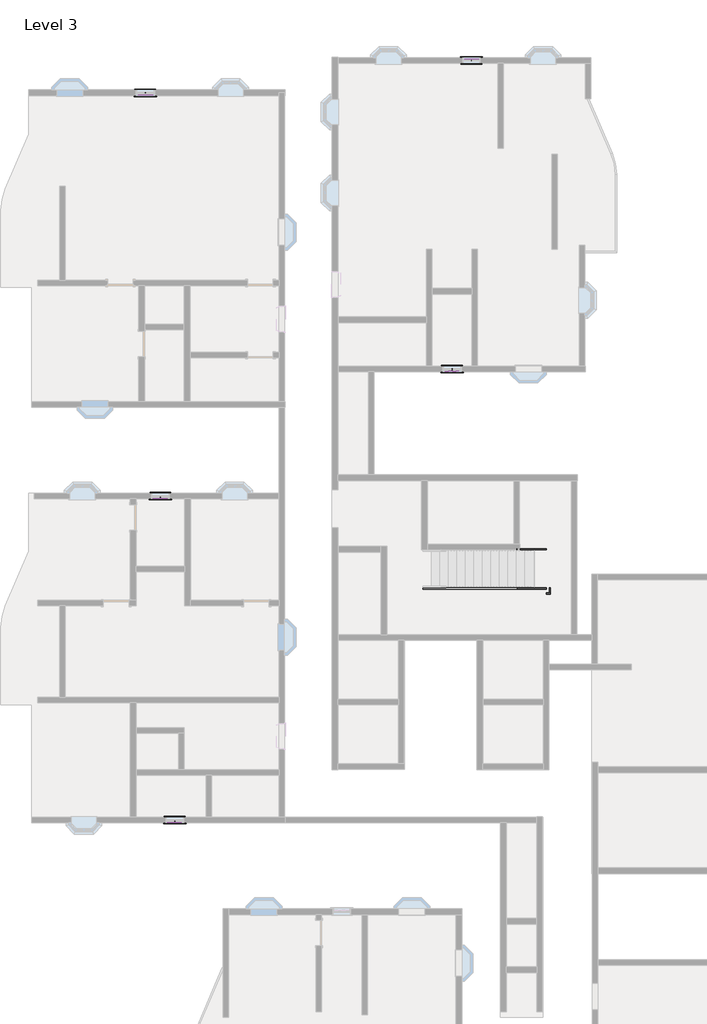
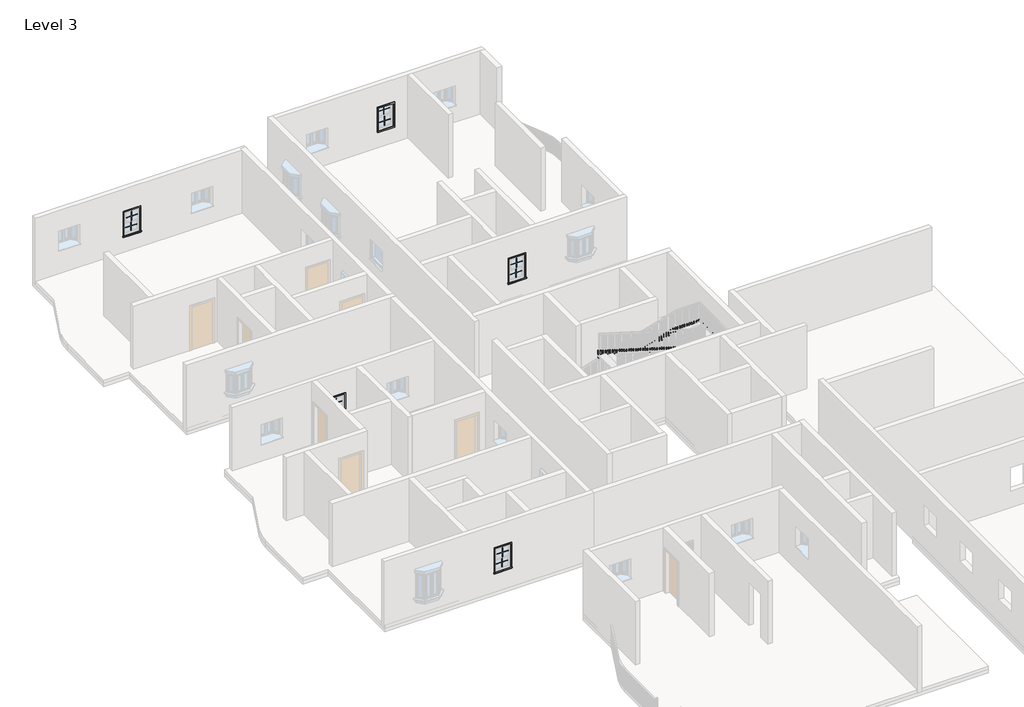
# One storey, part 14 of 14: 20 proxies, 6 members.
"""IFC4 building model written with IfcOpenShell, lengths in millimetres."""

from ifc_helpers import new_model, si_unit, frame, origin, place, context, project, spatial, polyline, outline, extrude, transform, mapped, element, save
from components import muntin_pattern_2x2_muntin_pattern_2x2_c35c595f, trim_window_exterior_flat_with_sill_e38017c9, trim_window_interior_flat_picture_frame_d728ed12

model = new_model("IFC4")

# Units and contexts
model_context = context("Model", 3, world=origin())
ifc_project = project(units=[si_unit("LENGTHUNIT", "METRE", prefix="MILLI")], contexts=[model_context])

# Site, building, storey
site = spatial("IfcSite", under=ifc_project)
building = spatial("IfcBuilding", under=site)
storey = spatial("IfcBuildingStorey", under=building, Name="Level 3", Elevation=6096.0)

# Proxies
placement = place(None, origin())
muntin_pattern_2x2_muntin_pattern_2x2_shape = muntin_pattern_2x2_muntin_pattern_2x2_c35c595f(model_context)
element("IfcBuildingElementProxy", 1, Name="Muntin Pattern_2x2 : Muntin Pattern_2x2", ObjectType="Muntin Pattern_2x2 : Muntin Pattern_2x2", at=placement, inside=storey, context=model_context, shape_type="MappedRepresentation", body=[
    mapped(muntin_pattern_2x2_muntin_pattern_2x2_shape, transform((-14639.3891351, 14368.0833494, 7566.025), x_axis=(-1.0, 0.0, 0.0), y_axis=(0.0, -1.0, 0.0), z_axis=(0.0, 0.0, 1.0))),
])
element("IfcBuildingElementProxy", 2, Name="Muntin Pattern_2x2 : Muntin Pattern_2x2", ObjectType="Muntin Pattern_2x2 : Muntin Pattern_2x2", at=placement, inside=storey, context=model_context, shape_type="MappedRepresentation", body=[
    mapped(muntin_pattern_2x2_muntin_pattern_2x2_shape, transform((-14639.3891351, 14412.5333494, 7086.6), x_axis=(-1.0, 0.0, 0.0), y_axis=(0.0, -1.0, 0.0), z_axis=(0.0, 0.0, 1.0))),
])
element("IfcBuildingElementProxy", 3, Name="Muntin Pattern_2x2 : Muntin Pattern_2x2", ObjectType="Muntin Pattern_2x2 : Muntin Pattern_2x2", at=placement, inside=storey, context=model_context, shape_type="MappedRepresentation", body=[
    mapped(muntin_pattern_2x2_muntin_pattern_2x2_shape, transform((-14125.0391351, 2785.6833494, 7566.025), x_axis=(-1.0, 0.0, 0.0), y_axis=(0.0, -1.0, 0.0), z_axis=(0.0, 0.0, 1.0))),
])
element("IfcBuildingElementProxy", 4, Name="Muntin Pattern_2x2 : Muntin Pattern_2x2", ObjectType="Muntin Pattern_2x2 : Muntin Pattern_2x2", at=placement, inside=storey, context=model_context, shape_type="MappedRepresentation", body=[
    mapped(muntin_pattern_2x2_muntin_pattern_2x2_shape, transform((-14125.0391351, 2830.1333494, 7086.6), x_axis=(-1.0, 0.0, 0.0), y_axis=(0.0, -1.0, 0.0), z_axis=(0.0, 0.0, 1.0))),
])
element("IfcBuildingElementProxy", 5, Name="Muntin Pattern_2x2 : Muntin Pattern_2x2", ObjectType="Muntin Pattern_2x2 : Muntin Pattern_2x2", at=placement, inside=storey, context=model_context, shape_type="MappedRepresentation", body=[
    mapped(muntin_pattern_2x2_muntin_pattern_2x2_shape, transform((-4206.3391351, 18910.0465905, 7566.025), x_axis=(-1.0, 0.0, 0.0), y_axis=(0.0, -1.0, 0.0), z_axis=(0.0, 0.0, 1.0))),
])
element("IfcBuildingElementProxy", 6, Name="Muntin Pattern_2x2 : Muntin Pattern_2x2", ObjectType="Muntin Pattern_2x2 : Muntin Pattern_2x2", at=placement, inside=storey, context=model_context, shape_type="MappedRepresentation", body=[
    mapped(muntin_pattern_2x2_muntin_pattern_2x2_shape, transform((-4206.3391351, 18954.4965905, 7086.6), x_axis=(-1.0, 0.0, 0.0), y_axis=(0.0, -1.0, 0.0), z_axis=(0.0, 0.0, 1.0))),
])
element("IfcBuildingElementProxy", 7, Name="Muntin Pattern_2x2 : Muntin Pattern_2x2", ObjectType="Muntin Pattern_2x2 : Muntin Pattern_2x2", at=placement, inside=storey, context=model_context, shape_type="MappedRepresentation", body=[
    mapped(muntin_pattern_2x2_muntin_pattern_2x2_shape, transform((-3514.1891351, 30066.9965905, 7566.025), x_axis=(1.0, 0.0, 0.0), y_axis=(0.0, 1.0, 0.0), z_axis=(0.0, 0.0, 1.0))),
])
element("IfcBuildingElementProxy", 8, Name="Muntin Pattern_2x2 : Muntin Pattern_2x2", ObjectType="Muntin Pattern_2x2 : Muntin Pattern_2x2", at=placement, inside=storey, context=model_context, shape_type="MappedRepresentation", body=[
    mapped(muntin_pattern_2x2_muntin_pattern_2x2_shape, transform((-3514.1891351, 30022.5465905, 7086.6), x_axis=(1.0, 0.0, 0.0), y_axis=(0.0, 1.0, 0.0), z_axis=(0.0, 0.0, 1.0))),
])
element("IfcBuildingElementProxy", 9, Name="Muntin Pattern_2x2 : Muntin Pattern_2x2", ObjectType="Muntin Pattern_2x2 : Muntin Pattern_2x2", at=placement, inside=storey, context=model_context, shape_type="MappedRepresentation", body=[
    mapped(muntin_pattern_2x2_muntin_pattern_2x2_shape, transform((-15175.9641351, 28782.5833494, 7566.025), x_axis=(-1.0, 0.0, 0.0), y_axis=(0.0, -1.0, 0.0), z_axis=(0.0, 0.0, 1.0))),
])
element("IfcBuildingElementProxy", 10, Name="Muntin Pattern_2x2 : Muntin Pattern_2x2", ObjectType="Muntin Pattern_2x2 : Muntin Pattern_2x2", at=placement, inside=storey, context=model_context, shape_type="MappedRepresentation", body=[
    mapped(muntin_pattern_2x2_muntin_pattern_2x2_shape, transform((-15175.9641351, 28827.0333494, 7086.6), x_axis=(-1.0, 0.0, 0.0), y_axis=(0.0, -1.0, 0.0), z_axis=(0.0, 0.0, 1.0))),
])
trim_window_exterior_flat_with_sill_shape = trim_window_exterior_flat_with_sill_e38017c9(model_context)
element("IfcBuildingElementProxy", 11, Name="Trim-Window-Exterior-Flat : with Sill", ObjectType="Trim-Window-Exterior-Flat : with Sill", at=placement, inside=storey, context=model_context, shape_type="MappedRepresentation", body=[
    mapped(trim_window_exterior_flat_with_sill_shape, transform((-14639.3891351, 14333.1583494, 8077.2), x_axis=(1.0, 0.0, 0.0), y_axis=(0.0, 0.0, 1.0), z_axis=(0.0, -1.0, 0.0))),
])
element("IfcBuildingElementProxy", 12, Name="Trim-Window-Exterior-Flat : with Sill", ObjectType="Trim-Window-Exterior-Flat : with Sill", at=placement, inside=storey, context=model_context, shape_type="MappedRepresentation", body=[
    mapped(trim_window_exterior_flat_with_sill_shape, transform((-14125.0391351, 2750.7583494, 8077.2), x_axis=(1.0, 0.0, 0.0), y_axis=(0.0, 0.0, 1.0), z_axis=(0.0, -1.0, 0.0))),
])
element("IfcBuildingElementProxy", 13, Name="Trim-Window-Exterior-Flat : with Sill", ObjectType="Trim-Window-Exterior-Flat : with Sill", at=placement, inside=storey, context=model_context, shape_type="MappedRepresentation", body=[
    mapped(trim_window_exterior_flat_with_sill_shape, transform((-4206.3391351, 18875.1215905, 8077.2), x_axis=(1.0, 0.0, 0.0), y_axis=(0.0, 0.0, 1.0), z_axis=(0.0, -1.0, 0.0))),
])
element("IfcBuildingElementProxy", 14, Name="Trim-Window-Exterior-Flat : with Sill", ObjectType="Trim-Window-Exterior-Flat : with Sill", at=placement, inside=storey, context=model_context, shape_type="MappedRepresentation", body=[
    mapped(trim_window_exterior_flat_with_sill_shape, transform((-3514.1891351, 30101.9215905, 8077.2), x_axis=(-1.0, 0.0, 0.0), y_axis=(0.0, 0.0, 1.0), z_axis=(0.0, 1.0, 0.0))),
])
element("IfcBuildingElementProxy", 15, Name="Trim-Window-Exterior-Flat : with Sill", ObjectType="Trim-Window-Exterior-Flat : with Sill", at=placement, inside=storey, context=model_context, shape_type="MappedRepresentation", body=[
    mapped(trim_window_exterior_flat_with_sill_shape, transform((-15175.9641351, 28747.6583494, 8077.2), x_axis=(1.0, 0.0, 0.0), y_axis=(0.0, 0.0, 1.0), z_axis=(0.0, -1.0, 0.0))),
])
trim_window_interior_flat_picture_frame_shape = trim_window_interior_flat_picture_frame_d728ed12(model_context)
element("IfcBuildingElementProxy", 16, Name="Trim-Window-Interior-Flat : Picture Frame", ObjectType="Trim-Window-Interior-Flat : Picture Frame", at=placement, inside=storey, context=model_context, shape_type="MappedRepresentation", body=[
    mapped(trim_window_interior_flat_picture_frame_shape, transform((-14639.3891351, 14536.3583494, 8077.2), x_axis=(-1.0, 0.0, 0.0), y_axis=(0.0, 0.0, 1.0), z_axis=(0.0, 1.0, 0.0))),
])
element("IfcBuildingElementProxy", 17, Name="Trim-Window-Interior-Flat : Picture Frame", ObjectType="Trim-Window-Interior-Flat : Picture Frame", at=placement, inside=storey, context=model_context, shape_type="MappedRepresentation", body=[
    mapped(trim_window_interior_flat_picture_frame_shape, transform((-14125.0391351, 2953.9583494, 8077.2), x_axis=(-1.0, 0.0, 0.0), y_axis=(0.0, 0.0, 1.0), z_axis=(0.0, 1.0, 0.0))),
])
element("IfcBuildingElementProxy", 18, Name="Trim-Window-Interior-Flat : Picture Frame", ObjectType="Trim-Window-Interior-Flat : Picture Frame", at=placement, inside=storey, context=model_context, shape_type="MappedRepresentation", body=[
    mapped(trim_window_interior_flat_picture_frame_shape, transform((-4206.3391351, 19078.3215905, 8077.2), x_axis=(-1.0, 0.0, 0.0), y_axis=(0.0, 0.0, 1.0), z_axis=(0.0, 1.0, 0.0))),
])
element("IfcBuildingElementProxy", 19, Name="Trim-Window-Interior-Flat : Picture Frame", ObjectType="Trim-Window-Interior-Flat : Picture Frame", at=placement, inside=storey, context=model_context, shape_type="MappedRepresentation", body=[
    mapped(trim_window_interior_flat_picture_frame_shape, transform((-3514.1891351, 29898.7215905, 8077.2), x_axis=(1.0, 0.0, 0.0), y_axis=(0.0, 0.0, 1.0), z_axis=(0.0, -1.0, 0.0))),
])
element("IfcBuildingElementProxy", 20, Name="Trim-Window-Interior-Flat : Picture Frame", ObjectType="Trim-Window-Interior-Flat : Picture Frame", at=placement, inside=storey, context=model_context, shape_type="MappedRepresentation", body=[
    mapped(trim_window_interior_flat_picture_frame_shape, transform((-15175.9641351, 28950.8583494, 8077.2), x_axis=(-1.0, 0.0, 0.0), y_axis=(0.0, 0.0, 1.0), z_axis=(0.0, 1.0, 0.0))),
])

# Members
element("IfcMember", 21, ObjectType="Stringer - 2\" Width", at=placement, inside=storey, context=model_context, shape_type="SweptSolid", body=[
    extrude(outline(polyline([(6287.5995961, -5254.0891351), (6096.0, -5254.0891351), (6096.0, -4832.019314), (7543.8, -6.019314), (7543.8, -1066.7544553), (6287.5995961, -5254.0891351)])), frame((0.0, 12506.0715905, 0.0), z_axis=(0.0, 1.0, 0.0), x_axis=(0.0, 0.0, 1.0)), (0.0, 0.0, 1.0), 50.8),
])
element("IfcMember", 22, ObjectType="Stringer - 2\" Width", at=placement, inside=storey, context=model_context, shape_type="SweptSolid", body=[
    extrude(outline(polyline([(54.5108649, 12556.8715905), (105.3108649, 12556.8715905), (105.3108649, 9478.4949943), (54.5108649, 9478.4949943), (54.5108649, 12556.8715905)])), frame((0.0, 0.0, 7239.0), z_axis=(0.0, 0.0, 1.0), x_axis=(1.0, 0.0, 0.0)), (0.0, 0.0, 1.0), 304.8),
])
element("IfcMember", 23, ObjectType="Stringer - 2\" Width", at=placement, inside=storey, context=model_context, shape_type="SweptSolid", body=[
    extrude(outline(polyline([(7239.0, 105.3108649), (7331.5395961, 105.3108649), (8939.3595961, -5254.0891351), (8621.1390537, -5254.0891351), (7239.0, -646.9589562), (7239.0, 105.3108649)])), frame((0.0, 9427.6949943, 0.0), z_axis=(0.0, 1.0, 0.0), x_axis=(0.0, 0.0, 1.0)), (0.0, 0.0, 1.0), 50.8),
])
element("IfcMember", 24, ObjectType="Stringer - 2\" Width", at=placement, inside=storey, context=model_context, shape_type="SweptSolid", body=[
    extrude(outline(polyline([(6287.5995961, -5254.0891351), (6096.0, -5254.0891351), (6096.0, -4832.019314), (7325.7390537, -732.8891351), (7543.8, -732.8891351), (7543.8, -1066.7544553), (6287.5995961, -5254.0891351)])), frame((0.0, 11103.4082924, 0.0), z_axis=(0.0, 1.0, 0.0), x_axis=(0.0, 0.0, 1.0)), (0.0, 0.0, 1.0), 50.8),
])
element("IfcMember", 25, ObjectType="Stringer - 2\" Width", at=placement, inside=storey, context=model_context, shape_type="SweptSolid", body=[
    extrude(outline(polyline([(-732.8891351, 11154.2082924), (-682.0891351, 11154.2082924), (-682.0891351, 10976.4082924), (-732.8891351, 10976.4082924), (-732.8891351, 11154.2082924)])), frame((0.0, 0.0, 7239.0), z_axis=(0.0, 0.0, 1.0), x_axis=(1.0, 0.0, 0.0)), (0.0, 0.0, 1.0), 304.8),
])
element("IfcMember", 26, ObjectType="Stringer - 2\" Width", at=placement, inside=storey, context=model_context, shape_type="SweptSolid", body=[
    extrude(outline(polyline([(7249.5390537, -682.0891351), (7567.7595961, -682.0891351), (8939.3595961, -5254.0891351), (8621.1390537, -5254.0891351), (7249.5390537, -682.0891351)])), frame((0.0, 10925.6082924, 0.0), z_axis=(0.0, 1.0, 0.0), x_axis=(0.0, 0.0, 1.0)), (0.0, 0.0, 1.0), 50.8),
])

save(model, "model.ifc")

# Revit data of these elements
# Type "Muntin Pattern_2x2 : Muntin Pattern_2x2"
#   Width [instance default] = 4' - 0"
#   Thickness = 0' - 0 1/2"
#   Height [instance default] = 4' - 0"
#   Distance = 0' - 0 3/4"
#   Interior Material [instance default] = none
#   Exterior Material [instance default] = none
#   Default Elevation = 0
# Type "Trim-Window-Exterior-Flat : with Sill"
#   Trim Width = 0' - 2 1/4"
#   Trim Thickness_Picture Frame = 0' - 1 1/4"
#   Trim Thickness_with Sill = 0' - 0 3/4"
#   Sill Thickness = 0' - 1 1/4"
#   Opening Width [instance default] = 2' - 0"
#   Opening Height [instance default] = 3' - 0"
#   Default Elevation = 4' - 0"
#   Sill = yes
#   Picture Frame = no
#   Trim Material [instance default] = none
# Type "Trim-Window-Interior-Flat : Picture Frame"
#   Trim Thickness_Picture Frame = 0' - 1 1/4"
#   Trim Width = 0' - 2 1/4"
#   Trim Thickness_with Sill = 0' - 0 3/4"
#   Sill Thickness = 0' - 1 1/4"
#   Opening Width [instance default] = 2' - 0"
#   Opening Height [instance default] = 3' - 0"
#   Default Elevation = 4' - 0"
#   Sill = no
#   Picture Frame = yes
#   Trim Material [instance default] = none
# Elements 1, 2, 3, 4, 5, 6, 7, 8, 9, 10 (IfcBuildingElementProxy, "Muntin Pattern_2x2 : Muntin Pattern_2x2")
#   Width = 1' - 8"
#   Height = 1' - 5 1/8"
#   Interior Material = Wood - Stained
#   Exterior Material = Clad - White
#   Phase Created = New Construction
#   Materials on its faces: "Clad - White", "Wood - Stained"
# Elements 11, 12, 13, 14, 15 (IfcBuildingElementProxy, "Trim-Window-Exterior-Flat : with Sill")
#   Opening Width = 2' - 2"
#   Opening Height = 3' - 6"
#   Trim Material = Clad - White
#   Phase Created = New Construction
#   Materials on its faces: "Clad - White"
# Elements 16, 17, 18, 19, 20 (IfcBuildingElementProxy, "Trim-Window-Interior-Flat : Picture Frame")
#   Opening Width = 2' - 2"
#   Opening Height = 3' - 6"
#   Trim Material = Wood - Stained
#   Phase Created = New Construction
#   Materials on its faces: "Wood - Stained"
# Elements 21, 22, 23, 24, 25, 26 (IfcMember, "Stringer - 2\" Width")
#   Phase Created = New Construction
# Materials
#   "Clad - White": class "Wood", colour RGB 242 242 238, transparency 0, Cost = 0
#   "Wood - Stained": class "Wood", colour RGB 224 178 126, transparency 0, Cost = 0
